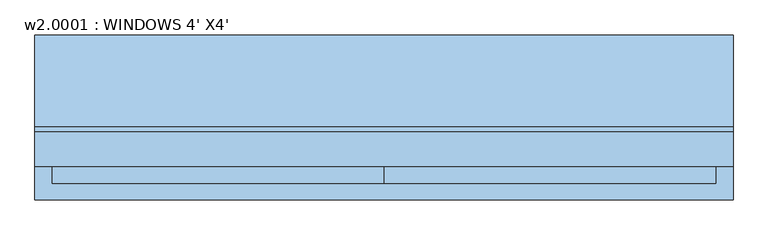
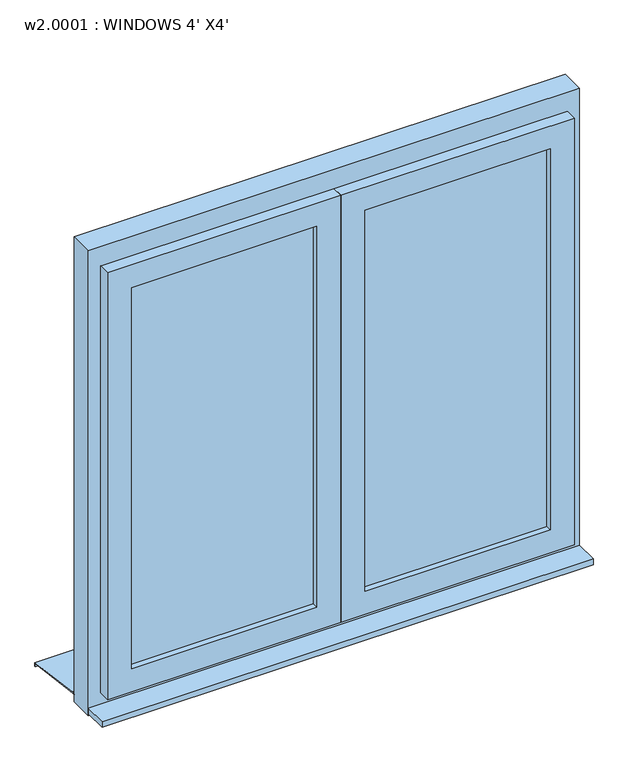
"""IFC4 building model written with IfcOpenShell, lengths in millimetres: window geometry, w2.0001 : WINDOWS 4' X4'."""

from ifc_helpers import new_model, si_unit, frame, origin, place, context, project, spatial, polyline, outline, extrude, faceted_brep, source, transform, mapped, element, save


def w2_0001_windows_4_x4_9dec5fc7(model_context):
    return source(origin(), model_context, "Body", "SolidModel", [
        extrude(outline(polyline([(-15.6778457, 1020.0), (144.3, 1000.0), (144.3, 990.0), (142.3, 990.0), (142.3, 998.3604634), (-15.8759277, 1018.0), (-25.7, 1018.0), (-25.7, 1020.0), (-15.6778457, 1020.0)])), frame((-609.6, 0.0, 0.0), z_axis=(1.0, 0.0, 0.0), x_axis=(0.0, 1.0, 0.0)), (0.0, 0.0, 1.0), 1219.2),
        extrude(outline(polyline([(-609.6, -144.3), (-609.6, -85.7), (609.6, -85.7), (609.6, -144.3), (-609.6, -144.3)])), frame((0.0, 0.0, 1005.0), z_axis=(0.0, 0.0, 1.0), x_axis=(1.0, 0.0, 0.0)), (0.0, 0.0, 1.0), 15.0),
        extrude(outline(polyline([(60.0, -70.7), (519.6, -70.7), (519.6, -100.7), (60.0, -100.7), (60.0, -70.7)])), frame((0.0, 0.0, 1110.0), z_axis=(0.0, 0.0, 1.0), x_axis=(1.0, 0.0, 0.0)), (0.0, 0.0, 1.0), 999.2),
        extrude(outline(polyline([(-519.6, -70.7), (-60.0, -70.7), (-60.0, -100.7), (-519.6, -100.7), (-519.6, -70.7)])), frame((0.0, 0.0, 1110.0), z_axis=(0.0, 0.0, 1.0), x_axis=(1.0, 0.0, 0.0)), (0.0, 0.0, 1.0), 999.2),
        extrude(outline(polyline([(2219.2, -609.6), (1000.0, -609.6), (1000.0, 609.6), (2219.2, 609.6), (2219.2, -609.6)]), holes=[polyline([(2139.2, -549.6), (2139.2, 549.6), (1080.0, 549.6), (1080.0, -549.6), (2139.2, -549.6)])]), frame((0.0, -85.7, 0.0), z_axis=(0.0, 1.0, 0.0), x_axis=(0.0, 0.0, 1.0)), (0.0, 0.0, 1.0), 60.0),
        extrude(outline(polyline([(30.0, -85.7), (-30.0, -85.7), (-30.0, -25.7), (30.0, -25.7), (30.0, -85.7)])), frame((0.0, 0.0, 1080.0), z_axis=(0.0, 0.0, 1.0), x_axis=(1.0, 0.0, 0.0)), (0.0, 0.0, 1.0), 1059.2),
        faceted_brep([(30.0, -85.7, 1080.0), (30.0, -55.7, 1080.0), (549.6, -55.7, 1080.0), (549.6, -85.7, 1080.0), (549.6, -55.7, 2139.2), (549.6, -85.7, 2139.2), (30.0, -55.7, 2139.2), (519.6, -55.7, 2109.2), (60.0, -55.7, 2109.2), (60.0, -55.7, 1110.0), (519.6, -55.7, 1110.0), (579.6, -85.7, 1050.0), (0.0, -85.7, 1050.0), (0.0, -85.7, 2169.2), (579.6, -85.7, 2169.2), (30.0, -85.7, 2139.2), (0.0, -115.7, 1050.0), (579.6, -115.7, 1050.0), (579.6, -115.7, 2169.2), (0.0, -115.7, 2169.2), (519.6, -115.7, 1110.0), (60.0, -115.7, 1110.0), (60.0, -115.7, 2109.2), (519.6, -115.7, 2109.2)], [[[0, 1, 2, 3]], [[3, 2, 4, 5]], [[2, 1, 6, 4], [7, 8, 9, 10]], [[11, 12, 13, 14], [5, 15, 0, 3]], [[16, 12, 11, 17]], [[17, 11, 14, 18]], [[18, 19, 16, 17], [20, 21, 22, 23]], [[9, 21, 20, 10]], [[10, 20, 23, 7]], [[15, 6, 1, 0]], [[19, 13, 12, 16]], [[8, 22, 21, 9]], [[5, 4, 6, 15]], [[18, 14, 13, 19]], [[7, 23, 22, 8]]]),
        faceted_brep([(-549.6, -85.7, 1080.0), (-549.6, -55.7, 1080.0), (-30.0, -55.7, 1080.0), (-30.0, -85.7, 1080.0), (-30.0, -55.7, 2139.2), (-30.0, -85.7, 2139.2), (-549.6, -55.7, 2139.2), (-60.0, -55.7, 2109.2), (-519.6, -55.7, 2109.2), (-519.6, -55.7, 1110.0), (-60.0, -55.7, 1110.0), (0.0, -85.7, 1050.0), (-579.6, -85.7, 1050.0), (-579.6, -85.7, 2169.2), (0.0, -85.7, 2169.2), (-549.6, -85.7, 2139.2), (-579.6, -115.7, 1050.0), (0.0, -115.7, 1050.0), (0.0, -115.7, 2169.2), (-579.6, -115.7, 2169.2), (-60.0, -115.7, 1110.0), (-519.6, -115.7, 1110.0), (-519.6, -115.7, 2109.2), (-60.0, -115.7, 2109.2)], [[[0, 1, 2, 3]], [[3, 2, 4, 5]], [[2, 1, 6, 4], [7, 8, 9, 10]], [[11, 12, 13, 14], [5, 15, 0, 3]], [[16, 12, 11, 17]], [[17, 11, 14, 18]], [[18, 19, 16, 17], [20, 21, 22, 23]], [[9, 21, 20, 10]], [[10, 20, 23, 7]], [[15, 6, 1, 0]], [[19, 13, 12, 16]], [[8, 22, 21, 9]], [[5, 4, 6, 15]], [[18, 14, 13, 19]], [[7, 23, 22, 8]]]),
    ])


if __name__ == "__main__":
    model = new_model("IFC4")
    model_context = context("Model", 3, world=origin())
    ifc_project = project(units=[si_unit("LENGTHUNIT", "METRE", prefix="MILLI")], contexts=[model_context])
    site = spatial("IfcSite", under=ifc_project)
    building = spatial("IfcBuilding", under=site)
    placement = place(None, origin())
    w2_0001_windows_4_x4_shape = w2_0001_windows_4_x4_9dec5fc7(model_context)
    element("IfcWindow", 1, ObjectType="w2.0001 : WINDOWS 4' X4'", at=placement, inside=building, context=model_context, shape_type="MappedRepresentation", body=[
        mapped(w2_0001_windows_4_x4_shape, transform((0.0, 0.0, 0.0), x_axis=(1.0, 0.0, 0.0), y_axis=(0.0, 1.0, 0.0), z_axis=(0.0, 0.0, 1.0))),
    ])
    save(model, "model.ifc")

# Revit data of these elements
# Type "w2.0001 : WINDOWS 4' X4'"
#   Type Mark = "22"
#   Operation = "DoublePanelVertical"
#   Keynote = "16.05.01"
#   Analytic Construction = "<None>"
#   Rough Width = 4' - 0"
#   Rough Height = 4' - 0"
#   Rahmentiefe = 0' - 2.3622"
#   Rahmenhöhe unten = 0' - 3.14961"
#   Rahmehöhe oben = 0' - 3.14961"
#   Rahmenbreite = 0' - 2.3622"
#   Height = 4' - 0"
#   Flügeltiefe = 0' - 2.3622"
#   Flügelbreite = 0' - 2.3622"
#   Einbautiefe (von außen) [instance default] = 0' - 5.51181"
#   Width = 4' - 0"
#   Kippflügel [instance default] = yes
#   Drehflügel im Grundriß darstellen [instance default] = no
#   Drehflügel [instance default] = yes
#   Define Thermal Properties by = 1
#   Rahmen [instance default] = none
#   Glas [instance default] = none
#   Flügel [instance default] = none
#   Fensterbank aussen [instance default] = none
#   Fensterbank innen [instance default] = none
#   Wall Closure = (empty or 0)
# Element 1 (IfcWindow, "w2.0001 : WINDOWS 4' X4'")
#   Materials on its faces: "Fenster - Kunststoff", "Fenster - Kunststoff weiss", "Glass", "Fenster - Holz"
# Materials
#   "Fenster - Kunststoff": colour RGB 249 249 249, transparency 0
#   "Fenster - Kunststoff weiss": colour RGB 249 249 249, transparency 0
#   "Glass": class "Glass", colour RGB 0 128 192, transparency 0.75, Description = "Soda Lime Glass", Cost = 0
#   "Fenster - Holz": colour RGB 216 135 75, transparency 0
